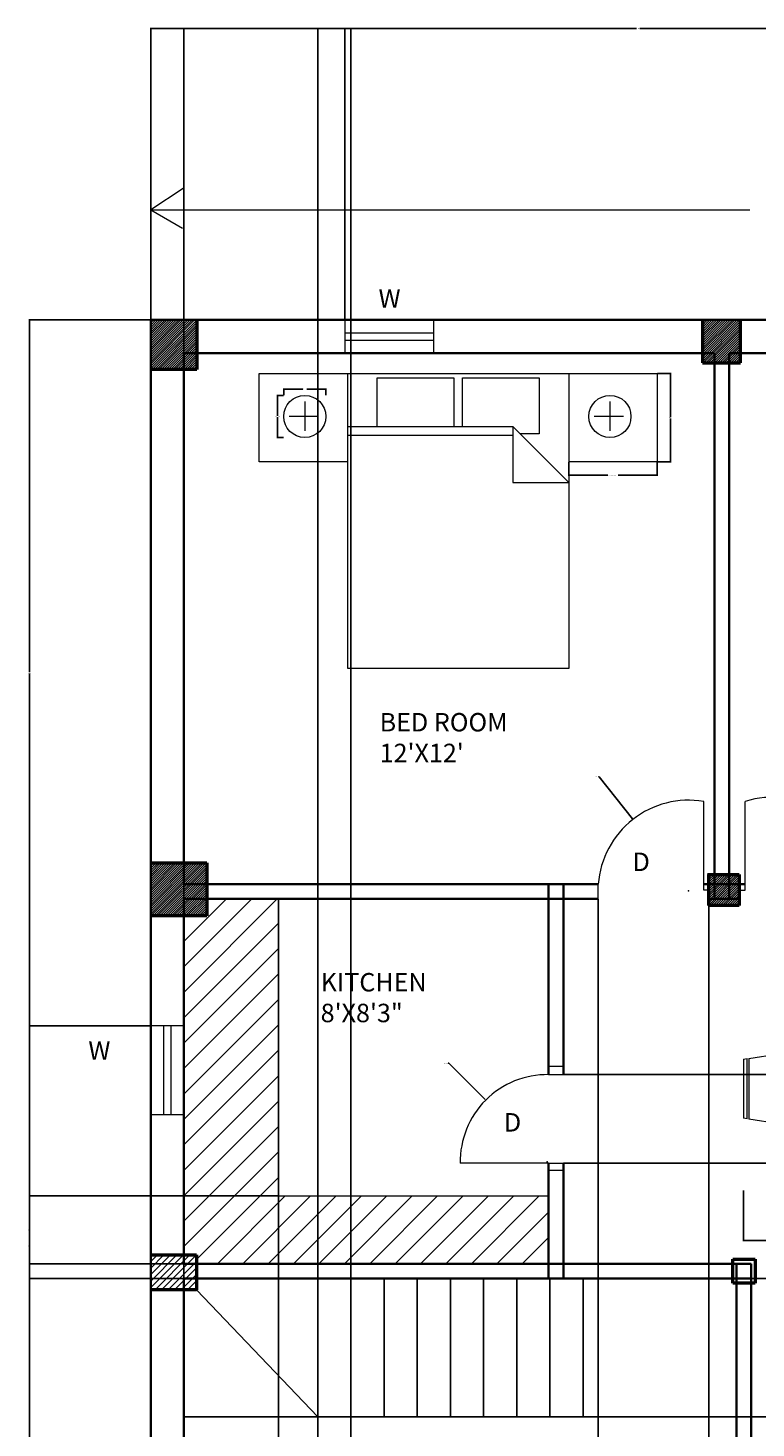
# Model space of a CAD drawing. Units: inches. Extents: x -12 to 472, y -585 to 99.
# Tile 2 of 4: x -12 to 186, y -281 to 99. Entities that reach past the tile are written whole.
import ezdxf

# ---------------------------------------------------------------- set-up
doc = ezdxf.new("R2010")
doc.units = ezdxf.units.IN
doc.header["$MEASUREMENT"] = 0
for name, color, linetype, lineweight in [('A-ANNO-DIMS', 2, 'Continuous', 18), ('A-ANNO-TEXT', 7, 'Continuous', 18), ('A-AREA-IDEN', 7, 'Continuous', 25), ('A-COLS', 7, 'Continuous', 50), ('A-COLS-PATT', 252, 'Continuous', 13), ('A-DOOR', 3, 'Continuous', 18), ('A-FLOR-FIXT', 9, 'Continuous', 20), ('A-FLOR-FIXT-PATT', 252, 'Continuous', 13), ('A-FLOR-STRS', 7, 'Continuous', 25), ('A-FURN', 8, 'Continuous', 18), ('A-GLAZ', 4, 'Continuous', 18), ('A-WALL', 7, 'Continuous', 35)]:
    doc.layers.add(name, color=color, linetype=linetype, lineweight=lineweight)
doc.styles.get("Standard").update_dxf_attribs({"font": 'arial.ttf'})
doc.dimstyles.get("Standard").update_dxf_attribs({"dimtxt": 0.18, "dimasz": 0.18, "dimexe": 0.18, "dimexo": 0.0625, "dimgap": 0.09, "dimtad": 0, "dimtih": 1, "dimtoh": 1, "dimdec": 4, "dimzin": 0, "dimdsep": 46, "dimtxsty": 'Standard', "dimcen": 0.09, "dimadec": 0, "dimazin": 0, "dimtfac": 1, "dimtdec": 4, "dimtofl": 0, "dimtmove": 0, "dimatfit": 3, "dimfxl": 1, "dimtolj": 1, "dimtzin": 0, "dimarcsym": 0})
pattern_1 = [(45, (-1281.90016, -702.76037), (-0.30935922, 0.30935922), [])]

# ---------------------------------------------------------------- blocks, each defined once
blk = doc.blocks.new('Bed - Queen')
for p, q in [((0, -80.00003), (0, 0)), ((0, 0), (59.99999, 0)), ((59.99999, 0), (59.99999, -80.00003)), ((7.99999, -1.2), (28.79998, -1.2)), ((7.99999, -14.4), (7.99999, -1.2)), ((28.79998, -1.2), (28.79998, -14.4)), ((31.19999, -1.2), (51.99999, -1.2)), ((31.19999, -14.4), (31.19999, -1.2)), ((51.99999, -1.2), (51.99999, -16.4)), ((0, -14.4), (44.8, -14.4)), ((59.99999, -29.6), (44.8, -14.4)), ((44.8, -14.4), (44.8, -29.6)), ((44.8, -16.8), (0, -16.8)), ((51.99999, -16.4), (46.79936, -16.4)), ((44.8, -29.6), (59.99999, -29.6)), ((59.99999, -80.00003), (0, -80.00003))]:
    blk.add_line(p, q)
blk = doc.blocks.new('Dining Set - 36 x 72 in.')
for p, q in [((-22, 27.5), (-22.1562, 26.50042)), ((-22, 27.5), (-6, 27.5)), ((-5.8437, 26.49966), (-6, 27.5)), ((6, 27.5), (5.8438, 26.50042)), ((6, 27.5), (22, 27.5)), ((22.1563, 26.49966), (22, 27.5)), ((-22.2343, 26.00059), (-23.4847, 17.99762)), ((-22.2304, 26), (-5.7608, 26)), ((-5.8416, 26.5), (-22.1534, 26.5)), ((-4.5152, 17.99762), (-5.7655, 25.99926)), ((5.7657, 26.00059), (4.5153, 17.99762)), ((5.7696, 26), (22.2392, 26)), ((22.1584, 26.5), (5.8466, 26.5)), ((23.4848, 17.99762), (22.2345, 25.99926)), ((36, 18), (-36, 18)), ((-36, 18), (-36, -18)), ((36, -18), (36, 18)), ((-45.5, 8), (-44.5004, 8.15617)), ((-45.5, 8), (-45.5, -8)), ((-44.5, -8.15843), (-44.5, 8.15338)), ((-44.0006, 8.23428), (-35.9976, 9.48474)), ((-44, 8.23041), (-44, -8.23915)), ((44.0006, 8.23428), (35.9976, 9.48474)), ((44, 8.23041), (44, -8.23915)), ((44.5, -8.15843), (44.5, 8.15338)), ((45.5, 8), (44.5005, 8.15617)), ((45.5, 8), (45.5, -8)), ((-44.4997, -8.15631), (-45.5, -8)), ((-35.9976, -9.48476), (-43.9993, -8.2345)), ((35.9976, -9.48476), (43.9993, -8.2345)), ((44.4997, -8.15631), (45.5, -8)), ((-36, -18), (36, -18)), ((-22.2343, -26.0006), (-23.4847, -17.99762)), ((-4.5152, -17.99762), (-5.7655, -25.99928)), ((5.7657, -26.0006), (4.5153, -17.99762)), ((23.4848, -17.99762), (22.2345, -25.99928)), ((-22.2304, -26), (-5.7608, -26)), ((-22, -27.5), (-22.1562, -26.50044)), ((-5.8416, -26.5), (-22.1534, -26.5)), ((-5.8437, -26.49967), (-6, -27.5)), ((5.7696, -26), (22.2392, -26)), ((6, -27.5), (5.8438, -26.50044)), ((22.1584, -26.5), (5.8466, -26.5)), ((22.1563, -26.49967), (22, -27.5)), ((-22, -27.5), (-6, -27.5)), ((6, -27.5), (22, -27.5))]:
    blk.add_line(p, q)
for points in [[(-36, 15), (-31.1772, 14.97754), (-26.8079, 14.91406), (-22.8538, 14.81543), (-19.276, 14.6875), (-16.0362, 14.53613), (-13.0957, 14.36718), (-10.4159, 14.18652), (-7.9583, 14), (-5.6904, 13.81315), (-3.6035, 13.63021), (-1.6954, 13.45508), (0.0365, 13.29166), (1.5945, 13.14388), (2.9811, 13.01562), (4.1988, 12.9108), (5.25, 12.83333), (6.1393, 12.78613), (6.8802, 12.76823), (7.4883, 12.77767), (7.9792, 12.8125), (8.3685, 12.87077), (8.6719, 12.95052), (8.9049, 13.0498), (9.0833, 13.16666), (9.2205, 13.29899), (9.3216, 13.44401), (9.3895, 13.59879), (9.4271, 13.76041), (9.4373, 13.92594), (9.4232, 14.09245), (9.3875, 14.257), (9.3333, 14.41666), (9.2638, 14.56917), (9.1836, 14.71484), (9.0975, 14.85465), (9.0104, 14.98958), (8.9272, 15.1206), (8.8529, 15.2487), (8.7922, 15.37483), (8.75, 15.5), (8.7305, 15.62467), (8.7344, 15.74739), (8.7617, 15.86621), (8.8125, 15.97916), (8.8867, 16.08431), (8.9844, 16.17968), (9.1055, 16.26334), (9.25, 16.33333), (9.4189, 16.38802), (9.6172, 16.42708), (9.8506, 16.45052), (10.125, 16.45833), (10.4463, 16.45052), (10.8203, 16.42708), (11.2529, 16.38802), (11.75, 16.33333), (12.3184, 16.26318), (12.9694, 16.17838), (13.7151, 16.07991), (14.5677, 15.96875), (15.5395, 15.84586), (16.6426, 15.71224), (17.8893, 15.56884), (19.2917, 15.41666), (20.859, 15.25667), (22.5879, 15.08984), (24.4721, 14.91715), (26.5052, 14.73958), (28.6809, 14.5581), (30.9929, 14.3737), (33.4347, 14.18733), (36, 14)], [(-36, 10), (-28.9766, 10.14274), (-23.1725, 10.20442), (-18.4241, 10.19775), (-14.5677, 10.13541), (-11.4399, 10.03011), (-8.877, 9.89453), (-6.7154, 9.74137), (-4.7917, 9.58333), (-2.9698, 9.43082), (-1.2246, 9.28515), (0.4415, 9.14534), (2.026, 9.01041), (3.5266, 8.87939), (4.9408, 8.7513), (6.266, 8.62516), (7.5, 8.5), (8.6411, 8.37549), (9.6914, 8.2539), (10.6538, 8.13818), (11.5312, 8.03125), (12.3267, 7.93603), (13.043, 7.85547), (13.6831, 7.79248), (14.25, 7.75), (14.7471, 7.7303), (15.1797, 7.73307), (15.5537, 7.75732), (15.875, 7.80208), (16.1494, 7.86637), (16.3828, 7.94922), (16.5811, 8.04964), (16.75, 8.16666), (16.8944, 8.29915), (17.0143, 8.44531), (17.1089, 8.60319), (17.1771, 8.77083), (17.218, 8.94629), (17.2305, 9.1276), (17.2137, 9.31282), (17.1667, 9.5), (17.0895, 9.6875), (16.987, 9.875), (16.8649, 10.0625), (16.7292, 10.25), (16.5856, 10.4375), (16.4401, 10.625), (16.2985, 10.8125), (16.1667, 11), (16.05, 11.18733), (15.9518, 11.3737), (15.8752, 11.5581), (15.8229, 11.73958), (15.798, 11.91715), (15.8034, 12.08984), (15.842, 12.25667), (15.9167, 12.41666), (16.0295, 12.56836), (16.1784, 12.70833), (16.3605, 12.83268), (16.5729, 12.9375), (16.8127, 13.01888), (17.0768, 13.07291), (17.3625, 13.0957), (17.6667, 13.08333), (17.9894, 13.03312), (18.3418, 12.94726), (18.7382, 12.82918), (19.1927, 12.68229), (19.7195, 12.51001), (20.3327, 12.31575), (21.0465, 12.10294), (21.875, 11.875), (22.8357, 11.63354), (23.959, 11.37304), (25.2786, 11.08618), (26.8282, 10.76562), (28.6414, 10.40405), (30.752, 9.99414), (33.1936, 9.52856), (36, 9)], [(-36, 5.5), (-30.7157, 5.3348), (-26.069, 5.20963), (-21.9946, 5.11767), (-18.4271, 5.05208), (-15.3009, 5.00602), (-12.5508, 4.97265), (-10.1112, 4.94515), (-7.9167, 4.91666), (-5.909, 4.88167), (-4.0586, 4.83984), (-2.3429, 4.79215), (-0.7396, 4.73958), (0.7739, 4.6831), (2.22, 4.6237), (3.6213, 4.56233), (5, 4.5), (6.373, 4.43782), (7.7344, 4.3776), (9.0723, 4.32129), (10.375, 4.27083), (11.6309, 4.22819), (12.8281, 4.19531), (13.9551, 4.17415), (15, 4.16666), (15.954, 4.17448), (16.819, 4.19791), (17.6001, 4.23698), (18.3021, 4.29166), (18.9299, 4.36198), (19.4883, 4.44791), (19.9823, 4.54948), (20.4167, 4.66666), (20.7969, 4.79899), (21.1302, 4.94401), (21.4245, 5.09879), (21.6875, 5.26041), (21.9271, 5.42594), (22.1511, 5.59245), (22.3672, 5.757), (22.5834, 5.91666), (22.8065, 6.06868), (23.0404, 6.21093), (23.2879, 6.34147), (23.5521, 6.45833), (23.8358, 6.55957), (24.142, 6.64323), (24.4735, 6.70735), (24.8334, 6.75), (25.2235, 6.76969), (25.642, 6.76692), (26.0858, 6.74267), (26.5521, 6.69791), (27.0379, 6.63362), (27.5404, 6.55078), (28.0565, 6.45036), (28.5834, 6.33333), (29.1242, 6.19987), (29.7071, 6.04687), (30.3661, 5.87044), (31.1354, 5.66666), (32.0493, 5.43164), (33.142, 5.16146), (34.4475, 4.85221), (36, 4.5)], [(-36, -1), (-30.7915, -0.6591), (-26.0195, -0.38216), (-21.6519, -0.16284), (-17.6563, 0.00521), (-14.0005, 0.12833), (-10.6523, 0.21289), (-7.5796, 0.26522), (-4.75, 0.29166), (-2.134, 0.29793), (0.2878, 0.28711), (2.5317, 0.26163), (4.6146, 0.22396), (6.5529, 0.17651), (8.3633, 0.12174), (10.0623, 0.06209), (11.6667, 0), (13.1899, -0.06201), (14.6341, -0.1211), (15.9982, -0.17432), (17.2813, -0.21875), (18.4823, -0.25147), (19.6003, -0.26953), (20.6343, -0.27002), (21.5834, -0.25), (22.4481, -0.20768), (23.2357, -0.14584), (23.9549, -0.06836), (24.6146, 0.02083), (25.2235, 0.11784), (25.7904, 0.21875), (26.3241, 0.31966), (26.8334, 0.41666), (27.3265, 0.50618), (27.8099, 0.58593), (28.2894, 0.65397), (28.7709, 0.70833), (29.2601, 0.74707), (29.763, 0.76823), (30.2855, 0.76985), (30.8334, 0.75), (31.4088, 0.70784), (31.9994, 0.64713), (32.589, 0.57275), (33.1615, 0.48958), (33.7008, 0.4025), (34.1908, 0.3164), (34.6153, 0.23616), (34.9584, 0.16666), (35.2099, 0.11165), (35.3848, 0.07031), (35.504, 0.04069), (35.5886, 0.02083), (35.6594, 0.00879), (35.7377, 0.0026), (35.8442, 0.00032), (36, 0)], [(-36, -6.5), (-27.1843, -6.31267), (-20.084, -6.1263), (-14.469, -5.9419), (-10.1094, -5.76042), (-6.7752, -5.58285), (-4.2363, -5.41016), (-2.2629, -5.24333), (-0.625, -5.08334), (0.8708, -4.93099), (2.2715, -4.78646), (3.5872, -4.64974), (4.8281, -4.52084), (6.0046, -4.39974), (7.127, -4.28646), (8.2053, -4.18099), (9.25, -4.08334), (10.2705, -3.99382), (11.2734, -3.91407), (12.2647, -3.84603), (13.25, -3.79167), (14.2354, -3.75293), (15.2266, -3.73177), (16.2295, -3.73015), (17.25, -3.75), (18.2912, -3.79248), (19.3451, -3.85547), (20.4009, -3.93604), (21.4479, -4.03125), (22.4754, -4.13819), (23.4727, -4.25391), (24.4289, -4.37549), (25.3334, -4.5), (26.1785, -4.62492), (26.9694, -4.74935), (27.7145, -4.87281), (28.4219, -4.99479), (29.1, -5.11483), (29.7572, -5.23242), (30.4016, -5.34709), (31.0417, -5.45834), (31.6837, -5.56437), (32.3262, -5.65821), (32.9658, -5.73153), (33.599, -5.77604), (34.2224, -5.78345), (34.8327, -5.74545), (35.4264, -5.65373), (36, -5.5)], [(-36, -10), (-26.4022, -9.81299), (-18.4675, -9.62891), (-11.9839, -9.45069), (-6.7396, -9.28125), (-2.5226, -9.12354), (0.8789, -8.98047), (3.6769, -8.85498), (6.0833, -8.75), (8.2767, -8.66765), (10.3021, -8.60677), (12.1712, -8.56543), (13.8958, -8.54167), (15.4876, -8.53353), (16.9583, -8.53907), (18.3197, -8.55632), (19.5834, -8.58334), (20.7616, -8.61841), (21.8685, -8.66081), (22.9188, -8.71004), (23.9271, -8.76563), (24.9081, -8.82707), (25.8763, -8.89388), (26.8465, -8.96558), (27.8334, -9.04167), (28.8474, -9.12118), (29.8828, -9.20117), (30.93, -9.27824), (31.9792, -9.34896), (33.0205, -9.40991), (34.0443, -9.45768), (35.0407, -9.48885), (36, -9.5)], [(-36, -14.5), (-30.0881, -14.33513), (-25.0332, -14.21224), (-20.7312, -14.12647), (-17.0781, -14.07292), (-13.97, -14.04671), (-11.3027, -14.04297), (-8.9724, -14.05681), (-6.875, -14.08334), (-4.9224, -14.11833), (-3.0905, -14.16016), (-1.3709, -14.20785), (0.2448, -14.26042), (1.7647, -14.3169), (3.1973, -14.3763), (4.5507, -14.43767), (5.8333, -14.5), (7.0554, -14.5621), (8.235, -14.62175), (9.3922, -14.67652), (10.5469, -14.72396), (11.7192, -14.76164), (12.929, -14.78711), (14.1965, -14.79794), (15.5417, -14.79167), (16.9933, -14.76424), (18.6152, -14.70508), (20.4804, -14.60197), (22.6615, -14.44271), (25.2312, -14.21509), (28.2624, -13.9069), (31.8277, -13.50594), (36, -13)]]:
    blk.add_lwpolyline(points)
blk = doc.blocks.new('WIN-24IN-EXT')
for p, q in [((0, 5.5), (24, 5.5)), ((0, 3.5), (24, 3.5))]:
    blk.add_line(p, q)
blk.add_lwpolyline([(0, 9), (24, 9), (24, 0), (0, 0)], close=True)
blk = doc.blocks.new('NIGHTSTAND-24IN')
for p, q in [((0, 24), (24, 24)), ((24, 24), (24, 0)), ((24, 0), (0, 0))]:
    blk.add_line(p, q)
blk = doc.blocks.new('LAMP-BEDSIDE-PLAN')
for p, q in [((5.72, 9.81), (5.72, 1.79)), ((1.49, 5.8), (9.4, 5.8))]:
    blk.add_line(p, q)
blk.add_circle((5.72, 5.72), 5.72)
blk = doc.blocks.new('*D14')
at = {"layer": 'A-ANNO-DIMS', "color": 0, "lineweight": -2, "transparency": 16777216}
for p, q in [((134.74, -18.94), (134.74, -22.66)), ((158.74, -18.94), (158.74, -22.66)), ((134.92, -22.48), (145.36, -22.48)), ((158.56, -22.48), (148.11, -22.48))]:
    blk.add_line(p, q, dxfattribs=at)
at = {"layer": 'A-ANNO-DIMS', "color": 0, "transparency": 16777216}
for points in [[(134.92, -22.45), (134.92, -22.51), (134.74, -22.48)], [(158.56, -22.45), (158.56, -22.51), (158.74, -22.48)]]:
    blk.add_solid(points, dxfattribs=at)
at = {"layer": 'Defpoints', "color": 0, "transparency": 16777216}
for p in [(134.74, -18.88), (158.74, -18.88), (158.74, -22.48)]:
    blk.add_point(p, dxfattribs=at)
at = {"layer": 'A-ANNO-DIMS', "color": 0, "transparency": 16777216, "insert": (146.74, -22.48), "char_height": 0.18, "attachment_point": 5}
blk.add_mtext('\\A1;NIGHTSTAND 24 TYP.', dxfattribs=at)
blk = doc.blocks.new('*D15')
at = {"layer": 'A-ANNO-DIMS', "color": 0, "lineweight": -2, "transparency": 16777216}
for p, q in [((158.8, 5.12), (162.52, 5.12)), ((162.34, 4.94), (162.34, -6.7)), ((162.34, -18.7), (162.34, -7.06)), ((158.8, -18.88), (162.52, -18.88))]:
    blk.add_line(p, q, dxfattribs=at)
at = {"layer": 'A-ANNO-DIMS', "color": 0, "transparency": 16777216}
for points in [[(162.31, 4.94), (162.37, 4.94), (162.34, 5.12)], [(162.31, -18.7), (162.37, -18.7), (162.34, -18.88)]]:
    blk.add_solid(points, dxfattribs=at)
at = {"layer": 'Defpoints', "color": 0, "transparency": 16777216}
for p in [(158.74, 5.12), (162.34, 5.12), (158.74, -18.88)]:
    blk.add_point(p, dxfattribs=at)
at = {"layer": 'A-ANNO-DIMS', "color": 0, "transparency": 16777216, "insert": (162.34, -6.88), "char_height": 0.18, "attachment_point": 5}
blk.add_mtext('\\A1;24 TYP.', dxfattribs=at)
blk = doc.blocks.new('*D16')
at = {"layer": 'A-ANNO-DIMS', "color": 0, "lineweight": -2, "transparency": 16777216}
for p, q in [((57.32, -0.84), (55.49, -0.84)), ((55.67, -1.02), (55.67, -6.37)), ((55.67, -12.09), (55.67, -6.73)), ((57.32, -12.27), (55.49, -12.27))]:
    blk.add_line(p, q, dxfattribs=at)
at = {"layer": 'A-ANNO-DIMS', "color": 0, "transparency": 16777216}
for points in [[(55.64, -1.02), (55.7, -1.02), (55.67, -0.84)], [(55.64, -12.09), (55.7, -12.09), (55.67, -12.27)]]:
    blk.add_solid(points, dxfattribs=at)
at = {"layer": 'Defpoints', "color": 0, "transparency": 16777216}
for p in [(55.67, -0.84), (57.38, -0.84), (57.38, -12.27)]:
    blk.add_point(p, dxfattribs=at)
at = {"layer": 'A-ANNO-DIMS', "color": 0, "transparency": 16777216, "insert": (55.67, -6.55), "char_height": 0.18, "attachment_point": 5}
blk.add_mtext('\\A1;LAMP 11 TYP.', dxfattribs=at)
blk = doc.blocks.new('*D17')
at = {"layer": 'A-ANNO-DIMS', "color": 0, "lineweight": -2, "transparency": 16777216}
for p, q in [((57.38, -0.77), (57.38, 1.06)), ((57.56, 0.88), (62.58, 0.88)), ((68.64, 0.88), (63.62, 0.88)), ((68.82, -0.77), (68.82, 1.06))]:
    blk.add_line(p, q, dxfattribs=at)
at = {"layer": 'A-ANNO-DIMS', "color": 0, "transparency": 16777216}
for points in [[(57.56, 0.91), (57.56, 0.85), (57.38, 0.88)], [(68.64, 0.91), (68.64, 0.85), (68.82, 0.88)]]:
    blk.add_solid(points, dxfattribs=at)
at = {"layer": 'Defpoints', "color": 0, "transparency": 16777216}
for p in [(68.82, 0.88), (57.38, -0.84), (68.82, -0.84)]:
    blk.add_point(p, dxfattribs=at)
at = {"layer": 'A-ANNO-DIMS', "color": 0, "transparency": 16777216, "insert": (63.1, 0.88), "char_height": 0.18, "attachment_point": 5}
blk.add_mtext('\\A1;11 TYP.', dxfattribs=at)
blk = doc.blocks.new('*D24')
at = {"layer": 'A-ANNO-DIMS', "color": 0, "lineweight": -2, "transparency": 16777216}
for p, q in [((182.14, -216.43), (182.14, -230.2)), ((273.14, -216.43), (273.14, -230.2)), ((182.32, -230.02), (226.97, -230.02)), ((272.96, -230.02), (228.31, -230.02))]:
    blk.add_line(p, q, dxfattribs=at)
at = {"layer": 'A-ANNO-DIMS', "color": 0, "transparency": 16777216}
for points in [[(182.32, -229.99), (182.32, -230.05), (182.14, -230.02)], [(272.96, -229.99), (272.96, -230.05), (273.14, -230.02)]]:
    blk.add_solid(points, dxfattribs=at)
at = {"layer": 'Defpoints', "color": 0, "transparency": 16777216}
for p in [(182.14, -216.37), (273.14, -216.37), (273.14, -230.02)]:
    blk.add_point(p, dxfattribs=at)
at = {"layer": 'A-ANNO-DIMS', "color": 0, "transparency": 16777216, "insert": (227.64, -230.02), "char_height": 0.18, "attachment_point": 5}
blk.add_mtext('\\A1;DINING 91', dxfattribs=at)
blk = doc.blocks.new('*D34')
at = {"layer": 'A-ANNO-DIMS', "color": 0, "lineweight": -2, "transparency": 16777216}
for p, q in [((30.22, -240.38), (-11.82, -240.38)), ((-11.64, -240.56), (-11.64, -301.7)), ((-11.64, -363.2), (-11.64, -302.06)), ((30.22, -363.38), (-11.82, -363.38))]:
    blk.add_line(p, q, dxfattribs=at)
at = {"layer": 'A-ANNO-DIMS', "color": 0, "transparency": 16777216}
for points in [[(-11.67, -240.56), (-11.61, -240.56), (-11.64, -240.38)], [(-11.67, -363.2), (-11.61, -363.2), (-11.64, -363.38)]]:
    blk.add_solid(points, dxfattribs=at)
at = {"layer": 'Defpoints', "color": 0, "transparency": 16777216}
for p in [(30.28, -240.38), (-11.64, -363.38), (30.28, -363.38)]:
    blk.add_point(p, dxfattribs=at)
at = {"layer": 'A-ANNO-DIMS', "color": 0, "transparency": 16777216, "insert": (-11.64, -301.88), "char_height": 0.18, "attachment_point": 5}
blk.add_mtext('\\A1;123', dxfattribs=at)
blk = doc.blocks.new('*D35')
at = {"layer": 'A-ANNO-DIMS', "color": 0, "lineweight": -2, "transparency": 16777216}
for p, q in [((30.28, -325.82), (30.28, 98.81)), ((66.61, -325.82), (66.61, 98.81)), ((30.46, 98.63), (47.98, 98.63)), ((66.43, 98.63), (48.91, 98.63))]:
    blk.add_line(p, q, dxfattribs=at)
at = {"layer": 'A-ANNO-DIMS', "color": 0, "transparency": 16777216}
for points in [[(30.46, 98.66), (30.46, 98.6), (30.28, 98.63)], [(66.43, 98.66), (66.43, 98.6), (66.61, 98.63)]]:
    blk.add_solid(points, dxfattribs=at)
at = {"layer": 'Defpoints', "color": 0, "transparency": 16777216}
for p in [(66.61, 98.63), (30.28, -325.88), (66.61, -325.88)]:
    blk.add_point(p, dxfattribs=at)
at = {"layer": 'A-ANNO-DIMS', "color": 0, "transparency": 16777216, "insert": (48.45, 98.63), "char_height": 0.18, "attachment_point": 5}
blk.add_mtext('\\A1;36.335', dxfattribs=at)
blk = doc.blocks.new('*D36')
at = {"layer": 'A-ANNO-DIMS', "color": 0, "lineweight": -2, "transparency": 16777216}
for p, q in [((66.61, -325.82), (66.61, 98.81)), ((75.61, -325.82), (75.61, 98.81)), ((66.79, 98.63), (70.96, 98.63)), ((75.43, 98.63), (71.26, 98.63))]:
    blk.add_line(p, q, dxfattribs=at)
at = {"layer": 'A-ANNO-DIMS', "color": 0, "transparency": 16777216}
for points in [[(66.79, 98.66), (66.79, 98.6), (66.61, 98.63)], [(75.43, 98.66), (75.43, 98.6), (75.61, 98.63)]]:
    blk.add_solid(points, dxfattribs=at)
at = {"layer": 'Defpoints', "color": 0, "transparency": 16777216}
for p in [(75.61, 98.63), (66.61, -325.88), (75.61, -325.88)]:
    blk.add_point(p, dxfattribs=at)
at = {"layer": 'A-ANNO-DIMS', "color": 0, "transparency": 16777216, "insert": (71.11, 98.63), "char_height": 0.18, "attachment_point": 5}
blk.add_mtext('\\A1;9', dxfattribs=at)
blk = doc.blocks.new('*D37')
at = {"layer": 'A-ANNO-DIMS', "color": 0, "lineweight": -2, "transparency": 16777216}
for p, q in [((138.68, -240.32), (471.69, -240.32)), ((471.51, -240.5), (471.51, -258.92)), ((471.51, -277.7), (471.51, -259.28)), ((138.68, -277.88), (471.69, -277.88))]:
    blk.add_line(p, q, dxfattribs=at)
at = {"layer": 'A-ANNO-DIMS', "color": 0, "transparency": 16777216}
for points in [[(471.48, -240.5), (471.54, -240.5), (471.51, -240.32)], [(471.48, -277.7), (471.54, -277.7), (471.51, -277.88)]]:
    blk.add_solid(points, dxfattribs=at)
at = {"layer": 'Defpoints', "color": 0, "transparency": 16777216}
for p in [(138.61, -240.32), (138.61, -277.88), (471.51, -277.88)]:
    blk.add_point(p, dxfattribs=at)
at = {"layer": 'A-ANNO-DIMS', "color": 0, "transparency": 16777216, "insert": (471.51, -259.1), "char_height": 0.18, "attachment_point": 5}
blk.add_mtext('\\A1;37.56', dxfattribs=at)
blk = doc.blocks.new('*D39')
at = {"layer": 'A-ANNO-DIMS', "color": 0, "lineweight": -2, "transparency": 16777216}
for p, q in [((142.75, -137.44), (142.75, -585.26)), ((172.75, -137.44), (172.75, -585.26)), ((142.93, -585.08), (157.53, -585.08)), ((172.57, -585.08), (157.97, -585.08))]:
    blk.add_line(p, q, dxfattribs=at)
at = {"layer": 'A-ANNO-DIMS', "color": 0, "transparency": 16777216}
for points in [[(142.93, -585.05), (142.93, -585.11), (142.75, -585.08)], [(172.57, -585.05), (172.57, -585.11), (172.75, -585.08)]]:
    blk.add_solid(points, dxfattribs=at)
at = {"layer": 'Defpoints', "color": 0, "transparency": 16777216}
for p in [(142.75, -137.38), (172.75, -137.38), (172.75, -585.08)]:
    blk.add_point(p, dxfattribs=at)
at = {"layer": 'A-ANNO-DIMS', "color": 0, "transparency": 16777216, "insert": (157.75, -585.08), "char_height": 0.18, "attachment_point": 5}
blk.add_mtext('\\A1;30', dxfattribs=at)
blk = doc.blocks.new('*D41')
at = {"layer": 'A-ANNO-DIMS', "color": 0, "lineweight": -2, "transparency": 16777216}
for p, q in [((21.28, 19.68), (21.28, 98.81)), ((74.01, 19.68), (74.01, 98.81)), ((21.46, 98.63), (47.25, 98.63)), ((73.83, 98.63), (48.04, 98.63))]:
    blk.add_line(p, q, dxfattribs=at)
at = {"layer": 'A-ANNO-DIMS', "color": 0, "transparency": 16777216}
for points in [[(21.46, 98.66), (21.46, 98.6), (21.28, 98.63)], [(73.83, 98.66), (73.83, 98.6), (74.01, 98.63)]]:
    blk.add_solid(points, dxfattribs=at)
at = {"layer": 'Defpoints', "color": 0, "transparency": 16777216}
for p in [(74.01, 98.63), (21.28, 19.62), (74.01, 19.62)]:
    blk.add_point(p, dxfattribs=at)
at = {"layer": 'A-ANNO-DIMS', "color": 0, "transparency": 16777216, "insert": (47.65, 98.63), "char_height": 0.18, "attachment_point": 5}
blk.add_mtext('\\A1;52.74', dxfattribs=at)
blk = doc.blocks.new('*D42')
at = {"layer": 'A-ANNO-DIMS', "color": 0, "lineweight": -2, "transparency": 16777216}
for p, q in [((74.01, 19.68), (74.01, 98.81)), ((233.15, 19.53), (233.15, 98.81)), ((74.19, 98.63), (153.13, 98.63)), ((232.97, 98.63), (154.04, 98.63))]:
    blk.add_line(p, q, dxfattribs=at)
at = {"layer": 'A-ANNO-DIMS', "color": 0, "transparency": 16777216}
for points in [[(74.19, 98.66), (74.19, 98.6), (74.01, 98.63)], [(232.97, 98.66), (232.97, 98.6), (233.15, 98.63)]]:
    blk.add_solid(points, dxfattribs=at)
at = {"layer": 'Defpoints', "color": 0, "transparency": 16777216}
for p in [(233.15, 98.63), (74.01, 19.62), (233.15, 19.47)]:
    blk.add_point(p, dxfattribs=at)
at = {"layer": 'A-ANNO-DIMS', "color": 0, "transparency": 16777216, "insert": (153.58, 98.63), "char_height": 0.18, "attachment_point": 5}
blk.add_mtext('\\A1;159.13', dxfattribs=at)
blk = doc.blocks.new('*D44')
at = {"layer": 'A-ANNO-DIMS', "color": 0, "lineweight": -2, "transparency": 16777216}
for p, q in [((30.28, -137.44), (30.28, -585.26)), ((55.95, -137.44), (55.95, -585.26)), ((30.46, -585.08), (42.65, -585.08)), ((55.77, -585.08), (43.58, -585.08))]:
    blk.add_line(p, q, dxfattribs=at)
at = {"layer": 'A-ANNO-DIMS', "color": 0, "transparency": 16777216}
for points in [[(30.46, -585.05), (30.46, -585.11), (30.28, -585.08)], [(55.77, -585.05), (55.77, -585.11), (55.95, -585.08)]]:
    blk.add_solid(points, dxfattribs=at)
at = {"layer": 'Defpoints', "color": 0, "transparency": 16777216}
for p in [(30.28, -137.38), (55.95, -137.38), (55.95, -585.08)]:
    blk.add_point(p, dxfattribs=at)
at = {"layer": 'A-ANNO-DIMS', "color": 0, "transparency": 16777216, "insert": (43.12, -585.08), "char_height": 0.18, "attachment_point": 5}
blk.add_mtext('\\A1;25.674', dxfattribs=at)
blk = doc.blocks.new('*D45')
at = {"layer": 'A-ANNO-DIMS', "color": 0, "lineweight": -2, "transparency": 16777216}
for p, q in [((55.89, -217.96), (-11.82, -217.96)), ((-11.64, -218.14), (-11.64, -226.99)), ((-11.64, -236.2), (-11.64, -227.35)), ((30.22, -236.38), (-11.82, -236.38))]:
    blk.add_line(p, q, dxfattribs=at)
at = {"layer": 'A-ANNO-DIMS', "color": 0, "transparency": 16777216}
for points in [[(-11.67, -218.14), (-11.61, -218.14), (-11.64, -217.96)], [(-11.67, -236.2), (-11.61, -236.2), (-11.64, -236.38)]]:
    blk.add_solid(points, dxfattribs=at)
at = {"layer": 'Defpoints', "color": 0, "transparency": 16777216}
for p in [(55.95, -217.96), (-11.64, -236.38), (30.28, -236.38)]:
    blk.add_point(p, dxfattribs=at)
at = {"layer": 'A-ANNO-DIMS', "color": 0, "transparency": 16777216, "insert": (-11.64, -227.17), "char_height": 0.18, "attachment_point": 5}
blk.add_mtext('\\A1;18.42', dxfattribs=at)
blk = doc.blocks.new('*D46')
at = {"layer": 'A-ANNO-DIMS', "color": 0, "lineweight": -2, "transparency": 16777216}
for p, q in [((133.34, -185.05), (471.69, -185.05)), ((471.51, -185.23), (471.51, -196.87)), ((471.51, -208.87), (471.51, -197.23)), ((133.34, -209.05), (471.69, -209.05))]:
    blk.add_line(p, q, dxfattribs=at)
at = {"layer": 'A-ANNO-DIMS', "color": 0, "transparency": 16777216}
for points in [[(471.48, -185.23), (471.54, -185.23), (471.51, -185.05)], [(471.48, -208.87), (471.54, -208.87), (471.51, -209.05)]]:
    blk.add_solid(points, dxfattribs=at)
at = {"layer": 'Defpoints', "color": 0, "transparency": 16777216}
for p in [(133.28, -185.05), (133.28, -209.05), (471.51, -209.05)]:
    blk.add_point(p, dxfattribs=at)
at = {"layer": 'A-ANNO-DIMS', "color": 0, "transparency": 16777216, "insert": (471.51, -197.05), "char_height": 0.18, "attachment_point": 5}
blk.add_mtext('\\A1;24', dxfattribs=at)
blk = doc.blocks.new('*D47')
at = {"layer": 'A-ANNO-DIMS', "color": 0, "lineweight": -2, "transparency": 16777216}
for p, q in [((21.22, 19.62), (-11.82, 19.62)), ((-11.64, 19.44), (-11.64, -75.93)), ((-11.64, -171.67), (-11.64, -76.3)), ((21.22, -171.85), (-11.82, -171.85))]:
    blk.add_line(p, q, dxfattribs=at)
at = {"layer": 'A-ANNO-DIMS', "color": 0, "transparency": 16777216}
for points in [[(-11.67, 19.44), (-11.61, 19.44), (-11.64, 19.62)], [(-11.67, -171.67), (-11.61, -171.67), (-11.64, -171.85)]]:
    blk.add_solid(points, dxfattribs=at)
at = {"layer": 'Defpoints', "color": 0, "transparency": 16777216}
for p in [(21.28, 19.62), (-11.64, -171.85), (21.28, -171.85)]:
    blk.add_point(p, dxfattribs=at)
at = {"layer": 'A-ANNO-DIMS', "color": 0, "transparency": 16777216, "insert": (-11.64, -76.12), "char_height": 0.18, "attachment_point": 5}
blk.add_mtext('\\A1;191.47', dxfattribs=at)
blk = doc.blocks.new('*D48')
at = {"layer": 'A-ANNO-DIMS', "color": 0, "lineweight": -2, "transparency": 16777216}
for p, q in [((21.22, -171.85), (-11.82, -171.85)), ((-11.64, -172.03), (-11.64, -231.32)), ((-11.64, -290.98), (-11.64, -231.69)), ((21.22, -291.16), (-11.82, -291.16))]:
    blk.add_line(p, q, dxfattribs=at)
at = {"layer": 'A-ANNO-DIMS', "color": 0, "transparency": 16777216}
for points in [[(-11.67, -172.03), (-11.61, -172.03), (-11.64, -171.85)], [(-11.67, -290.98), (-11.61, -290.98), (-11.64, -291.16)]]:
    blk.add_solid(points, dxfattribs=at)
at = {"layer": 'Defpoints', "color": 0, "transparency": 16777216}
for p in [(21.28, -171.85), (-11.64, -291.16), (21.28, -291.16)]:
    blk.add_point(p, dxfattribs=at)
at = {"layer": 'A-ANNO-DIMS', "color": 0, "transparency": 16777216, "insert": (-11.64, -231.51), "char_height": 0.18, "attachment_point": 5}
blk.add_mtext('\\A1;119.3', dxfattribs=at)
blk = doc.blocks.new('*D55')
at = {"layer": 'A-ANNO-DIMS', "color": 0, "lineweight": -2, "transparency": 16777216}
for p, q in [((142.83, -104.25), (143.01, -104.25)), ((143.01, -104.25), (151.99, -115.71)), ((167.15, -135.19), (167.33, -135.19)), ((167.24, -135.28), (167.24, -135.1))]:
    blk.add_line(p, q, dxfattribs=at)
at = {"layer": 'A-ANNO-DIMS', "color": 0, "transparency": 16777216}
blk.add_solid([(152.01, -115.7), (151.97, -115.73), (152.1, -115.86)], dxfattribs=at)
at = {"layer": 'Defpoints', "color": 0, "transparency": 16777216}
for p in [(152.1, -115.86), (167.24, -135.19)]:
    blk.add_point(p, dxfattribs=at)
at = {"layer": 'A-ANNO-DIMS', "color": 0, "transparency": 16777216, "insert": (142.36, -104.25), "char_height": 0.18, "attachment_point": 5}
blk.add_mtext('\\A1;R24.56', dxfattribs=at)
blk = doc.blocks.new('*D56')
at = {"layer": 'A-ANNO-DIMS', "color": 0, "lineweight": -2, "transparency": 16777216}
for p, q in [((101.99, -181.94), (102.17, -181.94)), ((102.17, -181.94), (112.06, -191.83)), ((128.8, -208.66), (128.98, -208.66)), ((128.89, -208.75), (128.89, -208.57))]:
    blk.add_line(p, q, dxfattribs=at)
at = {"layer": 'A-ANNO-DIMS', "color": 0, "transparency": 16777216}
blk.add_solid([(112.08, -191.81), (112.04, -191.85), (112.19, -191.96)], dxfattribs=at)
at = {"layer": 'Defpoints', "color": 0, "transparency": 16777216}
for p in [(112.19, -191.96), (128.89, -208.66)]:
    blk.add_point(p, dxfattribs=at)
at = {"layer": 'A-ANNO-DIMS', "color": 0, "transparency": 16777216, "insert": (101.44, -181.94), "char_height": 0.18, "attachment_point": 5}
blk.add_mtext('\\A1;R23.613', dxfattribs=at)

msp = doc.modelspace()

# ---------------------------------------------------------------- hatches: boundary and pattern name
at = {"layer": 'A-COLS-PATT'}
h = msp.add_hatch(dxfattribs=at)
h.set_pattern_fill('ANSI31', color=256, scale=3.5)
h.set_pattern_definition(pattern_1)
h.paths.add_polyline_path([(181.3779, 19.6212), (171.004, 19.6212), (171.004, 10.6212), (174.2783, 10.6212), (174.2783, 7.9633), (178.2783, 7.9633), (178.2783, 10.6212), (181.3779, 10.6212)])
h.paths.add_polyline_path([(181.3779, 10.6212), (178.2783, 10.6212), (178.2783, 7.9633), (181.3779, 7.9633)])
h.paths.add_polyline_path([(174.2783, 10.6212), (171.004, 10.6212), (171.004, 7.9633), (174.2783, 7.9633)])
h.paths.add_polyline_path([(33.7842, 19.6212), (21.2783, 19.6212), (21.2783, 6.2301), (30.2783, 6.2301), (30.2783, 10.6212), (33.7842, 10.6212)])
h.paths.add_polyline_path([(33.7842, 10.6212), (30.2783, 10.6212), (30.2783, 6.2301), (33.7842, 6.2301)], flags=17)
h = msp.add_hatch(dxfattribs=at)
h.set_pattern_fill('ANSI31', color=256, scale=3.5)
h.set_pattern_definition(pattern_1)
h.paths.add_polyline_path([(36.5249, -133.3788), (30.2783, -133.3788), (30.2783, -127.5805), (21.2783, -127.5805), (21.2783, -142.0038), (30.2783, -142.0038), (30.2783, -137.3788), (36.5249, -137.3788)])
h.paths.add_polyline_path([(36.5249, -127.5805), (30.2783, -127.5805), (30.2783, -133.3788), (36.5249, -133.3788)], flags=17)
h.paths.add_polyline_path([(36.5249, -137.3788), (30.2783, -137.3788), (30.2783, -142.0038), (36.5249, -142.0038)], flags=17)
h = msp.add_hatch(dxfattribs=at)
h.set_pattern_fill('ANSI31', color=256, scale=3.5)
h.set_pattern_definition(pattern_1)
h.paths.add_polyline_path([(178.2783, -133.3788), (174.2783, -133.3788), (174.2783, -137.3788), (178.2783, -137.3788)])
h.paths.add_polyline_path([(178.2783, -130.763), (174.2783, -130.763), (174.2783, -133.3788), (178.2783, -133.3788)])
h.paths.add_polyline_path([(174.2783, -130.763), (172.7504, -130.763), (172.7504, -133.3788), (174.2783, -133.3788)])
h.paths.add_polyline_path([(174.2783, -133.3788), (172.7504, -133.3788), (172.7504, -137.3788), (174.2783, -137.3788)])
h.paths.add_polyline_path([(181.0026, -137.3788), (172.7504, -137.3788), (172.7504, -139.195), (181.0026, -139.195)])
h.paths.add_polyline_path([(181.0026, -133.3788), (178.2783, -133.3788), (178.2783, -137.3788), (181.0026, -137.3788)])
h.paths.add_polyline_path([(181.0026, -130.763), (178.2783, -130.763), (178.2783, -133.3788), (181.0026, -133.3788)])
h.paths.add_polyline_path([(381.2783, -128.4288), (372.2783, -128.4288), (372.2783, -133.3788), (367.5282, -133.3788), (367.5282, -137.3788), (372.2783, -137.3788), (372.2783, -141.3418), (381.2783, -141.3418)])
h.paths.add_polyline_path([(372.2783, -128.4288), (367.5282, -128.4288), (367.5282, -133.3788), (372.2783, -133.3788)])
h.paths.add_polyline_path([(372.2783, -137.3788), (367.5282, -137.3788), (367.5282, -141.3418), (372.2783, -141.3418)], flags=17)
h.paths.add_polyline_path([(316.2734, -130.7939), (306.1194, -130.7939), (306.1194, -133.3788), (316.2734, -133.3788)])
h.paths.add_polyline_path([(312.2783, -133.3788), (308.2783, -133.3788), (308.2783, -137.3788), (312.2783, -137.3788)])
h.paths.add_polyline_path([(316.2734, -133.3788), (312.2783, -133.3788), (312.2783, -137.3788), (316.2734, -137.3788)])
h.paths.add_polyline_path([(316.2734, -137.3788), (312.2783, -137.3788), (312.2783, -140.1848), (316.2734, -140.1848)])
h.paths.add_polyline_path([(312.2783, -137.3788), (308.2783, -137.3788), (308.2783, -140.1848), (312.2783, -140.1848)])
h.paths.add_polyline_path([(308.2783, -137.3788), (306.1194, -137.3788), (306.1194, -140.1848), (308.2783, -140.1848)])
h.paths.add_polyline_path([(308.2783, -133.3788), (306.1194, -133.3788), (306.1194, -137.3788), (308.2783, -137.3788)])
h = msp.add_hatch(dxfattribs=at)
h.set_pattern_fill('ANSI31', color=256, scale=10)
h.set_pattern_definition([(45, (-1281.9002, -702.7604), (-0.8838835, 0.8838835), [])])
h.paths.add_polyline_path([(33.6941, -236.3788), (30.2783, -236.3788), (30.2783, -233.9155), (21.2783, -233.9155), (21.2783, -243.3987), (30.2783, -243.3987), (30.2783, -240.3788), (33.6941, -240.3788)])
h.paths.add_polyline_path([(33.6941, -233.9155), (30.2783, -233.9155), (30.2783, -236.3788), (33.6941, -236.3788)], flags=17)
h.paths.add_polyline_path([(33.6941, -240.3788), (30.2783, -240.3788), (30.2783, -243.3987), (33.6941, -243.3987)], flags=17)
at = {"layer": 'A-FLOR-FIXT-PATT'}
h = msp.add_hatch(dxfattribs=at)
h.set_pattern_fill('ANSI31', color=256, scale=39)
h.set_pattern_definition([(45, (-1281.9, -702.7604), (-3.447146, 3.447146), [])])
h.paths.add_polyline_path([(55.9524, -137.3788), (36.5249, -137.3788), (36.5249, -142.0038), (30.2783, -142.0038), (30.2783, -233.9155), (33.6941, -233.9155), (33.6941, -236.3788), (129.2783, -236.3788), (129.2783, -217.9596), (55.9524, -217.9596)])

# ---------------------------------------------------------------- linework, layer by layer
at = {"layer": 'A-ANNO-DIMS'}
for p, q in [((21.2783, 35.2691), (21.2783, 63.6755)), ((30.0885, 55.293), (21.2783, 49.4723)), ((21.2783, 49.4723), (183.8983, 49.4723)), ((21.2783, 49.4723), (29.9269, 44.4791))]:
    msp.add_line(p, q, dxfattribs=at)
at = {"layer": 'A-COLS'}
for p, q in [((33.7842, 19.6212), (33.7842, 6.2301)), ((171.004, 19.6212), (171.004, 7.9633)), ((181.3779, 7.9633), (181.3779, 19.6212)), ((171.004, 7.9633), (181.3779, 7.9633)), ((33.7842, 6.2301), (21.2783, 6.2301)), ((21.2783, -127.5805), (36.5249, -127.5805)), ((36.5249, -127.5805), (36.5249, -142.0038)), ((172.371, -130.763), (181.0026, -130.763)), ((172.7504, -139.195), (172.7504, -130.763)), ((181.0026, -130.763), (181.0026, -139.195)), ((181.0026, -139.195), (172.7504, -139.195)), ((36.5249, -142.0038), (21.2783, -142.0038)), ((21.2783, -233.9155), (33.6941, -233.9155)), ((33.6941, -233.9155), (33.6941, -243.3987)), ((179.2537, -241.6274), (179.2537, -235.0561)), ((179.2537, -235.0561), (179.3772, -235.0561)), ((179.3772, -235.0561), (185.3076, -235.0561)), ((185.3076, -235.0561), (185.3076, -241.6274)), ((185.3076, -241.6274), (179.2537, -241.6274)), ((33.6941, -243.3987), (21.2783, -243.3987))]:
    msp.add_line(p, q, dxfattribs=at)
at = {"layer": 'A-DOOR'}
for p, q in [((171.3526, -134.979), (171.3526, -110.979)), ((182.597, -134.979), (182.597, -110.979)), ((142.7504, -137.3788), (142.7504, -133.3788)), ((172.7504, -134.979), (171.3526, -134.979)), ((181.0026, -134.979), (182.597, -134.979)), ((129.2783, -182.7659), (133.2783, -182.7659)), ((129.2783, -185.0467), (133.2783, -185.0467)), ((129.2783, -209.0467), (105.2783, -209.0467)), ((129.2783, -209.0467), (133.2783, -209.0467)), ((129.2783, -210.9228), (133.2783, -210.9228))]:
    msp.add_line(p, q, dxfattribs=at)
for centre, radius, start, end in [((189.4395, -131.5126), 21.6437, 355.053745, 108.429724), ((167.2426, -135.1919), 24.5592, 80.366369, 175.766205), ((128.888, -208.6564), 23.613, 89.053022, 180.946978)]:
    msp.add_arc(centre, radius, start, end, dxfattribs=at)
at = {"layer": 'A-FLOR-FIXT'}
for p, q in [((55.9524, -137.3788), (55.9524, -217.9596)), ((55.9524, -217.9596), (129.2783, -217.9596))]:
    msp.add_line(p, q, dxfattribs=at)
at = {"layer": 'A-FLOR-STRS'}
for p, q in [((66.6133, -240.3222), (66.6133, -363.3788)), ((75.6133, -240.3222), (75.6133, -277.8788)), ((84.6133, -240.3222), (84.6133, -277.8788)), ((93.6133, -240.3222), (93.6133, -277.8788)), ((102.6133, -240.3222), (102.6133, -277.8788)), ((111.6133, -240.3222), (111.6133, -277.8788)), ((120.6133, -240.3222), (120.6133, -277.8788)), ((129.6133, -240.3222), (129.6133, -277.8788)), ((138.6133, -240.3222), (138.6133, -277.8788)), ((33.6941, -243.3987), (66.6133, -277.8788)), ((30.2783, -277.8788), (180.2783, -277.8788))]:
    msp.add_line(p, q, dxfattribs=at)
at = {"layer": 'A-WALL'}
for p, q in [((30.2783, 10.6212), (174.2783, 10.6212)), ((30.2783, -133.3788), (30.2783, 10.6212)), ((174.2783, -137.3788), (174.2783, 10.6212)), ((178.2783, -137.3788), (178.2783, 10.6212)), ((178.2783, 10.6212), (326.2783, 10.6212)), ((30.2783, -133.3788), (142.7504, -133.3788)), ((129.2783, -185.0467), (129.2783, -133.3788)), ((133.2783, -185.0467), (133.2783, -133.3788)), ((171.3526, -133.3788), (182.597, -133.3788)), ((30.2783, -137.3788), (142.7504, -137.3788)), ((30.2783, -236.3788), (30.2783, -137.3788)), ((172.7504, -137.3788), (181.0026, -137.3788)), ((129.2783, -240.3788), (129.2783, -209.0467)), ((133.2783, -240.3788), (133.2783, -209.0467)), ((30.2783, -236.3788), (184.2783, -236.3788)), ((180.2783, -337.6735), (180.2783, -236.3788)), ((184.2783, -337.6735), (184.2783, -236.3788)), ((30.2783, -240.3788), (184.2783, -240.3788)), ((30.2783, -363.3788), (30.2783, -240.3788))]:
    msp.add_line(p, q, dxfattribs=at)
msp.add_lwpolyline([(21.2783, 19.6212), (381.2783, 19.6212), (381.2783, -526.3788), (21.2783, -526.3788)], close=True, dxfattribs=at)

# ---------------------------------------------------------------- block references
at = {"layer": 'A-FURN', "rotation": 180}
msp.add_blockref('NIGHTSTAND-24IN', (74.7389, 5.1244), dxfattribs=at)
at = {"layer": 'A-FURN'}
for name, p in [('Bed - Queen', (74.739, 5.1242)), ('NIGHTSTAND-24IN', (134.739, -18.876)), ('LAMP-BEDSIDE-PLAN', (57.381, -12.272)), ('LAMP-BEDSIDE-PLAN', (140.187, -12.272)), ('Dining Set - 36 x 72 in.', (227.6392, -188.8665))]:
    msp.add_blockref(name, p, dxfattribs=at)
at = {"layer": 'A-GLAZ'}
msp.add_blockref('WIN-24IN-EXT', (74.014, 10.621), dxfattribs=at)
at = {"layer": 'A-GLAZ', "extrusion": (0, 0, -1), "zscale": -1, "rotation": 269.9999999999999}
msp.add_blockref('WIN-24IN-EXT', (-30.2785, -171.853), dxfattribs=at)

# ---------------------------------------------------------------- texts
at = {"layer": 'A-ANNO-TEXT', "char_height": 5, "attachment_point": 1}
for s, width, insert in [('W', 41.793086, (83.1078, 27.9637)), ('D', 12.206964, (152.053, -124.8279)), ('W', 16.914769, (4.3635, -176.0009)), ('D', 15.015921, (117.134, -195.4866))]:
    msp.add_mtext_dynamic_manual_height_columns(s, width=width, gutter_width=25, heights=[0], dxfattribs=dict(at, insert=insert))
at = {"layer": 'A-AREA-IDEN', "char_height": 5, "attachment_point": 1}
for s, width, insert in [("BED ROOM\\P12'X12'", 94.921965, (83.4116, -86.9717)), ('KITCHEN\\P8\'X8\'3"', 40.503104, (67.4068, -157.4897))]:
    msp.add_mtext_dynamic_manual_height_columns(s, width=width, gutter_width=25, heights=[0], dxfattribs=dict(at, insert=insert))

# ---------------------------------------------------------------- dimensions: what is measured, and where the dimension line sits
at = {"layer": 'A-ANNO-DIMS'}
for base, p1, p2, override, picture, middle in [((74.0143, 98.6273), (21.2783, 19.6212), (74.0143, 19.6212), {"dimdec": 2, "dimlfac": 1, "dimrnd": 0, "dimzin": 0, "dimdsep": 46, "dimlunit": 2}, '*D41', (47.6463, 98.6273)), ((66.6133, 98.6273), (30.2783, -325.8788), (66.6133, -325.8788), {"dimdec": 3, "dimlfac": 1, "dimrnd": 0, "dimzin": 0, "dimdsep": 46, "dimlunit": 2}, '*D35', (48.4458, 98.6273)), ((75.6133, 98.6273), (66.6133, -325.8788), (75.6133, -325.8788), {"dimdec": 0, "dimlfac": 1, "dimrnd": 0, "dimzin": 0, "dimdsep": 46, "dimlunit": 2}, '*D36', (71.1133, 98.6273)), ((233.1482, 98.6273), (74.0143, 19.6212), (233.1482, 19.468), {"dimdec": 2, "dimlfac": 1, "dimrnd": 0, "dimzin": 0, "dimdsep": 46, "dimlunit": 2}, '*D42', (153.5813, 98.6273)), ((55.9524, -585.0813), (30.2783, -137.3788), (55.9524, -137.3788), {"dimdec": 3, "dimlfac": 1, "dimrnd": 0, "dimzin": 0, "dimdsep": 46, "dimlunit": 2}, '*D44', (43.1153, -585.0813)), ((172.7504, -585.0813), (142.7504, -137.3788), (172.7504, -137.3788), {"dimdec": 0, "dimlfac": 1, "dimrnd": 0, "dimzin": 0, "dimdsep": 46, "dimlunit": 2}, '*D39', (157.7504, -585.0813))]:
    dim = msp.add_linear_dim(base=base, p1=p1, p2=p2, dimstyle='Standard', override=override, dxfattribs=at)
    dim.commit()
    dim.dimension.update_dxf_attribs({"geometry": picture, "text_midpoint": middle})
for base, p1, p2, override, picture, middle in [((-11.6441, -171.8533), (21.2783, 19.6212), (21.2783, -171.8533), {"dimdec": 2, "dimlfac": 1, "dimrnd": 0, "dimzin": 0, "dimdsep": 46, "dimlunit": 2}, '*D47', (-11.6441, -76.116)), ((-11.6441, -291.1587), (21.2783, -171.8533), (21.2783, -291.1587), {"dimdec": 1, "dimlfac": 1, "dimrnd": 0, "dimzin": 0, "dimdsep": 46, "dimlunit": 2}, '*D48', (-11.6441, -231.506)), ((471.5096, -209.0467), (133.2783, -185.0467), (133.2783, -209.0467), {"dimdec": 0, "dimlfac": 1, "dimrnd": 0, "dimzin": 0, "dimdsep": 46, "dimlunit": 2}, '*D46', (471.5096, -197.0467)), ((-11.6441, -236.3788), (55.9524, -217.9596), (30.2783, -236.3788), {"dimdec": 2, "dimlfac": 1, "dimrnd": 0, "dimzin": 0, "dimdsep": 46, "dimlunit": 2}, '*D45', (-11.6441, -227.1692)), ((-11.6441, -363.3788), (30.2783, -240.3788), (30.2783, -363.3788), {"dimdec": 0, "dimlfac": 1, "dimrnd": 0, "dimzin": 0, "dimdsep": 46, "dimlunit": 2}, '*D34', (-11.6441, -301.8788)), ((471.5096, -277.8788), (138.6133, -240.3222), (138.6133, -277.8788), {"dimdec": 2, "dimlfac": 1, "dimrnd": 0, "dimzin": 0, "dimdsep": 46, "dimlunit": 2}, '*D37', (471.5096, -259.1005))]:
    dim = msp.add_linear_dim(base=base, p1=p1, p2=p2, angle=90, dimstyle='Standard', override=override, dxfattribs=at)
    dim.commit()
    dim.dimension.update_dxf_attribs({"geometry": picture, "text_midpoint": middle})
for base, p1, p2, text, picture, middle in [((162.339, 5.1242), (158.739, -18.8758), (158.739, 5.1242), '<> TYP.', '*D15', (162.339, -6.8758)), ((55.666, -0.8365), (57.3813, -12.2718), (57.3813, -0.8365), 'LAMP <> TYP.', '*D16', (55.666, -6.5542))]:
    dim = msp.add_linear_dim(base=base, p1=p1, p2=p2, angle=90, text=text, dimstyle='Standard', override={"dimdec": 0, "dimlfac": 1, "dimrnd": 0, "dimzin": 0, "dimdsep": 46, "dimlunit": 2}, dxfattribs=at)
    dim.commit()
    dim.dimension.update_dxf_attribs({"geometry": picture, "text_midpoint": middle})
for base, p1, p2, text, picture, middle in [((68.8166, 0.8788), (57.3813, -0.8365), (68.8166, -0.8365), '<> TYP.', '*D17', (63.099, 0.8788)), ((158.739, -22.4758), (134.739, -18.8758), (158.739, -18.8758), 'NIGHTSTAND <> TYP.', '*D14', (146.739, -22.4758)), ((273.1392, -230.0165), (182.1392, -216.3665), (273.1392, -216.3665), 'DINING <>', '*D24', (227.6392, -230.0165))]:
    dim = msp.add_linear_dim(base=base, p1=p1, p2=p2, text=text, dimstyle='Standard', override={"dimdec": 0, "dimlfac": 1, "dimrnd": 0, "dimzin": 0, "dimdsep": 46, "dimlunit": 2}, dxfattribs=at)
    dim.commit()
    dim.dimension.update_dxf_attribs({"geometry": picture, "text_midpoint": middle})
for center, mpoint, override, picture, middle in [((167.2426, -135.1919), (152.1003, -115.8563), {"dimdec": 2, "dimlfac": 1, "dimrnd": 0, "dimzin": 0, "dimdsep": 46, "dimlunit": 2}, '*D55', (142.355, -104.255)), ((128.888, -208.6564), (112.1908, -191.9598), {"dimdec": 3, "dimlfac": 1, "dimrnd": 0, "dimzin": 0, "dimdsep": 46, "dimlunit": 2}, '*D56', (101.4428, -181.9419))]:
    dim = msp.add_radius_dim(center=center, mpoint=mpoint, dimstyle='Standard', override=override, dxfattribs=at)
    dim.commit()
    dim.dimension.update_dxf_attribs({"geometry": picture, "text_midpoint": middle, "dimtype": 164})

doc.saveas('drawing.dxf')
